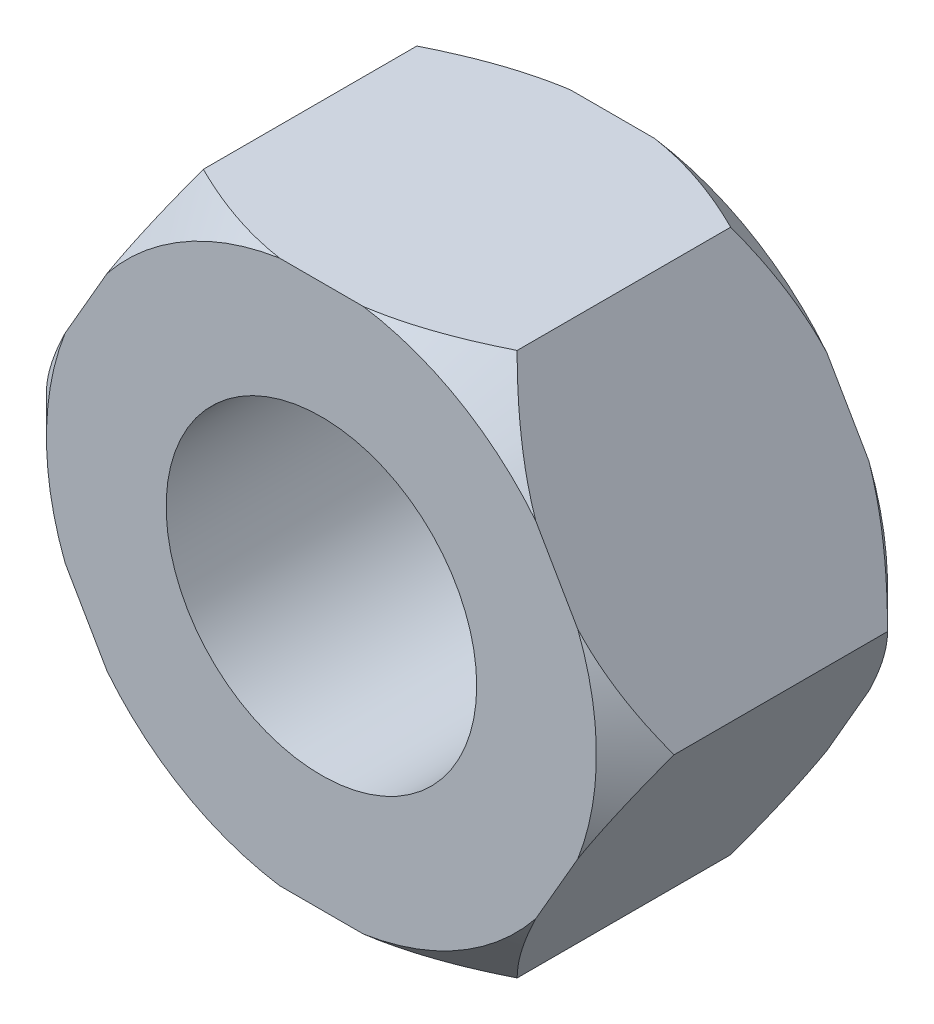
SolidWorks part; units mm, degrees
material "Plain Carbon Steel"
ref_plane "Front Plane" through (0, 0, 0) normal (0, 0, 1) x (1, 0, 0)
ref_plane "Top Plane" through (0, 0, 0) normal (0, 1, 0) x (1, 0, 0)
ref_plane "Right Plane" through (0, 0, 0) normal (1, 0, 0) x (0, 0, -1)
sketch "Hex Profile 28 AF" plane through (0, 0, 0) normal (0, 0, 1) x (1, 0, 0)
  line L0 (-243.7839, 0) -> (11945.4116, 0) construction
  line L1 (0, -243.7839) -> (0, 11945.4116) construction
  line L3 (16.1658, 0) -> (8.0829, 14)
  line L4 (8.0829, 14) -> (-8.0829, 14)
  line L5 (-8.0829, 14) -> (-16.1658, 0)
  line L6 (-16.1658, 0) -> (-8.0829, -14)
  line L7 (-8.0829, -14) -> (8.0829, -14)
  line L8 (8.0829, -14) -> (16.1658, 0)
  circle A0 centre (0, 0) radius 14 construction
  dimension "D1" = 28
extrude "Hex Body 15 Thick" add sketch "Hex Profile 28 AF" along normal mid plane 15
sketch "Bore Profile Ø16" plane through (0, 0, 0) normal (0, 0, 1) x (1, 0, 0)
  circle A0 centre (0, 0) radius 8
  dimension "D1" = 16
extrude "Bore Ø16 Thru" cut sketch "Bore Profile Ø16" against normal mid plane 15
sketch "Chamfer Profile 2mm" plane through (0, 0, 0) normal (0, 1, 0) x (1, 0, 0)
  line L0 (-1000, 0) -> (49000, 0) construction
  line L1 (0, -1000) -> (0, 49000) construction
  line L3 (16.1658, 7.5) -> (16.1658, 5.5)
  line L4 (16.1658, -7.5) -> (16.1658, 7.5) construction
  line L5 (16.1658, 5.5) -> (14.1658, 7.5)
  line L6 (16.1658, 7.5) -> (8.0829, 7.5) construction
  line L7 (14.1658, 7.5) -> (16.1658, 7.5)
  line L8 (16.1658, -7.5) -> (16.1658, -5.5)
  line L9 (16.1658, -5.5) -> (14.1658, -7.5)
  line L10 (16.1658, -7.5) -> (8.0829, -7.5) construction
  line L11 (14.1658, -7.5) -> (16.1658, -7.5)
  dimension "D1" = 2
  dimension "D2" = 2
  dimension "D3" = 2
  dimension "D4" = 2
revolve "Double-Sided Chamfer 2mm" cut sketch "Chamfer Profile 2mm" angle 360 about L1
